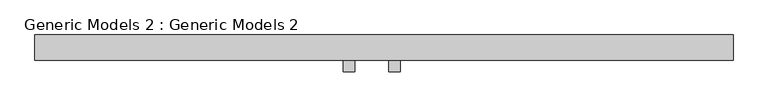
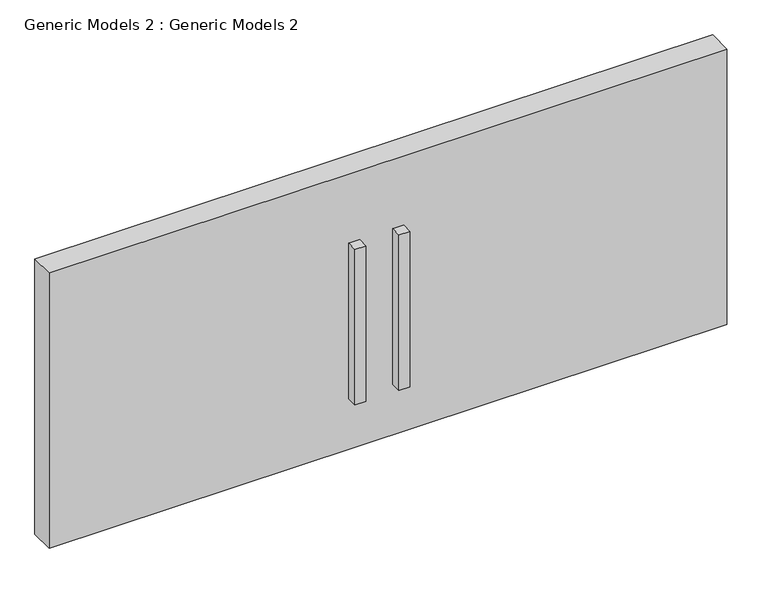
"""IFC4 building model written with IfcOpenShell, lengths in millimetres: proxy geometry, Generic Models 2 : Generic Models 2."""

from ifc_helpers import new_model, si_unit, frame, origin, place, context, project, spatial, polyline, outline, extrude, source, transform, mapped, element, save


def generic_models_2_generic_models_2_568ed07e(model_context):
    return source(origin(), model_context, "Body", "SweptSolid", [
        extrude(outline(polyline([(-4858.9900592, 515.0055142), (-4909.7900592, 515.0055142), (-4909.7900592, 565.8055142), (-4858.9900592, 565.8055142), (-4858.9900592, 515.0055142)])), frame((0.0, 0.0, 552.6438765), z_axis=(0.0, 0.0, 1.0), x_axis=(1.0, 0.0, 0.0)), (0.0, 0.0, 1.0), 762.0),
        extrude(outline(polyline([(-4655.7900592, 515.0055142), (-4706.5900592, 515.0055142), (-4706.5900592, 565.8055142), (-4655.7900592, 565.8055142), (-4655.7900592, 515.0055142)])), frame((0.0, 0.0, 552.6438765), z_axis=(0.0, 0.0, 1.0), x_axis=(1.0, 0.0, 0.0)), (0.0, 0.0, 1.0), 762.0),
        extrude(outline(polyline([(-6296.2569651, 680.1055142), (-3159.3569651, 680.1055142), (-3159.3569651, 565.8055142), (-6296.2569651, 565.8055142), (-6296.2569651, 680.1055142)])), frame((0.0, 0.0, 304.8), z_axis=(0.0, 0.0, 1.0), x_axis=(1.0, 0.0, 0.0)), (0.0, 0.0, 1.0), 1348.2575529),
    ])


if __name__ == "__main__":
    model = new_model("IFC4")
    model_context = context("Model", 3, world=origin())
    ifc_project = project(units=[si_unit("LENGTHUNIT", "METRE", prefix="MILLI")], contexts=[model_context])
    site = spatial("IfcSite", under=ifc_project)
    building = spatial("IfcBuilding", under=site)
    placement = place(None, origin())
    generic_models_2_generic_models_2_shape = generic_models_2_generic_models_2_568ed07e(model_context)
    element("IfcBuildingElementProxy", 1, Name="Generic Models 2 : Generic Models 2", ObjectType="Generic Models 2 : Generic Models 2", at=placement, inside=building, context=model_context, shape_type="MappedRepresentation", body=[
        mapped(generic_models_2_generic_models_2_shape, transform((0.0, 0.0, 0.0), x_axis=(1.0, 0.0, 0.0), y_axis=(0.0, 1.0, 0.0), z_axis=(0.0, 0.0, 1.0))),
    ])
    save(model, "model.ifc")

# Revit data of these elements
# Element 1 (IfcBuildingElementProxy, "Generic Models 2 : Generic Models 2")
#   Materials on its faces: "1 wall brown", "1 wall white"
# Materials
#   "1 wall brown": class "Generic", colour RGB 61 46 37, transparency 0, Cost = 0
#   "1 wall white": class "Generic", colour RGB 244 245 241, transparency 0, Cost = 0
